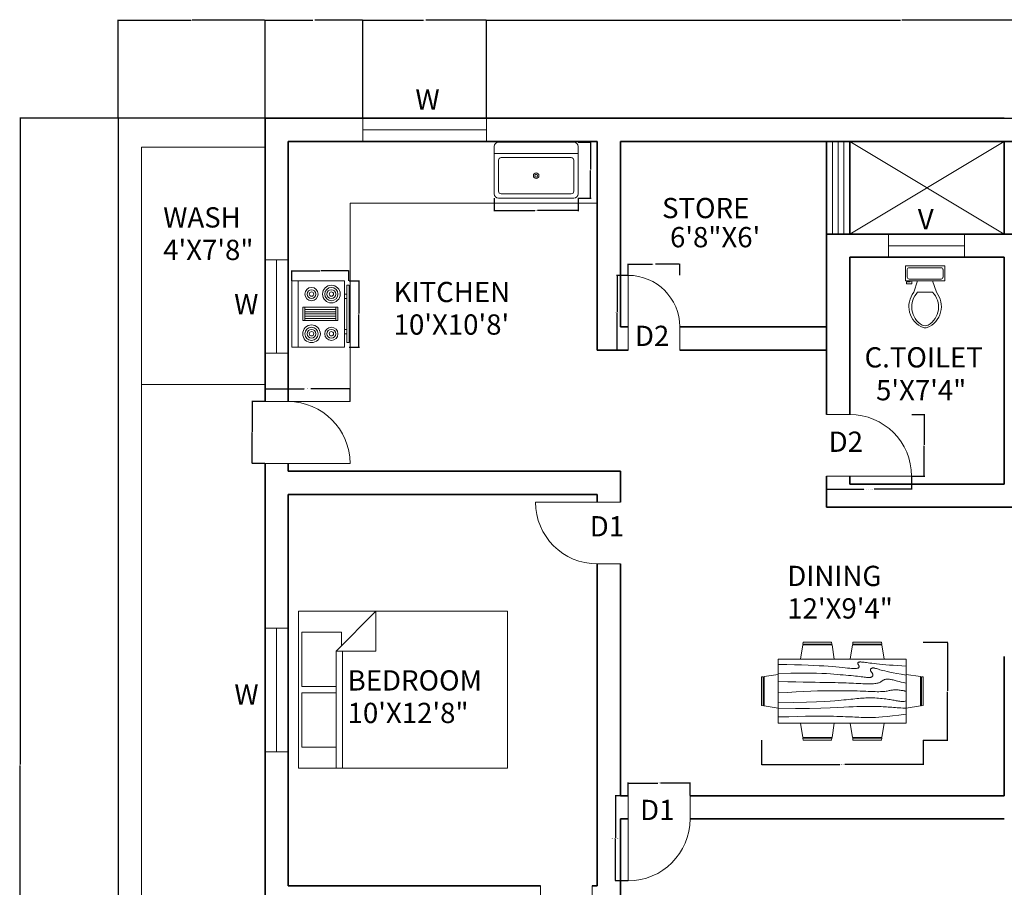
# Model space of a CAD drawing. Units: feet. Extents: x 2219 to 3039, y 1768 to 2369.
# Tile 2 of 16: x 2219 to 2601, y 2032 to 2369. Entities that reach past the tile are written whole.
import ezdxf

# ---------------------------------------------------------------- set-up
doc = ezdxf.new("R2010")
doc.units = ezdxf.units.FT
for name, color, linetype, lineweight in [('A-ANNO-DIMS', 2, 'Continuous', 18), ('A-ANNO-TEXT', 7, 'Continuous', 18), ('A-AREA-IDEN', 7, 'Continuous', 18), ('A-DOOR', 4, 'Continuous', 20), ('A-EQPM', 9, 'Continuous', 18), ('A-FLOR-CASE', 9, 'Continuous', 20), ('A-FLOR-FIXT', 9, 'Continuous', 18), ('A-FLOR-OPEN', 8, 'Continuous', 13), ('A-FURN', 8, 'Continuous', 18), ('A-GLAZ', 4, 'Continuous', 18), ('A-WALL', 7, 'Continuous', 35), ('C-PROP', 7, 'Continuous', 30), ('C-SITE', 3, 'Continuous', 20)]:
    doc.layers.add(name, color=color, linetype=linetype, lineweight=lineweight)
doc.styles.get("Standard").update_dxf_attribs({"font": 'arial.ttf'})
doc.dimstyles.get("Standard").update_dxf_attribs({"dimtxt": 0.18, "dimasz": 0.18, "dimexe": 0.18, "dimexo": 0.0625, "dimgap": 0.09, "dimtad": 0, "dimtih": 1, "dimtoh": 1, "dimdec": 4, "dimzin": 0, "dimdsep": 46, "dimtxsty": 'Standard', "dimcen": 0.09, "dimadec": 0, "dimazin": 0, "dimtfac": 1, "dimtdec": 4, "dimtofl": 0, "dimtmove": 0, "dimatfit": 3, "dimfxl": 1, "dimtolj": 1, "dimtzin": 0, "dimarcsym": 0})

# ---------------------------------------------------------------- blocks, each defined once
blk = doc.blocks.new('Toilet - top')
for p, q in [((9.5, -6), (9.5, -2)), ((-10, -8.5), (-8, -8.5)), ((-10, -9.5), (-10, -8.5)), ((-7, -9.5), (-10, -9.5)), ((-8, -8.5), (-8, -8)), ((-7, -8), (-7, -9.5)), ((-4, -8), (-6, -14)), ((4, -8), (6, -14)), ((4, -14), (-4, -14))]:
    blk.add_line(p, q)
blk.add_lwpolyline([(10.5, -8), (10.5, 0), (-10.5, 0), (-10.5, -8)], close=True)
for points in [[(-9.5, -2), (-9.5, -6)], [(8.5, -1), (-8.5, -1)], [(-8.5, -7), (8.5, -7)]]:
    blk.add_lwpolyline(points)
for centre, radius, start, end in [((-8.62, -1.88), 0.884, 81.8699, 188.1301), ((8.62, -1.88), 0.884, 351.8699, 98.1301), ((-8.62, -6.12), 0.884, 171.8699, 278.1301), ((8.62, -6.12), 0.884, 261.8699, 8.1301), ((3.52, -21.58), 12.17, 141.4691, 247.9714), ((4.2, -21.82), 11.33, 136.3677, 238.9468), ((-3.52, -21.58), 12.17, 292.0284, 38.5307), ((-4.2, -21.82), 11.33, 301.053, 43.6321), ((0, -27.88), 4, 245.7318, 294.2682), ((0, -29), 4, 254.8605, 285.1395)]:
    blk.add_arc(centre, radius, start, end)
blk = doc.blocks.new('Bed - Queen')
for p, q in [((0, -80.00003), (0, 0)), ((0, 0), (59.99999, 0)), ((59.99999, 0), (59.99999, -80.00003)), ((7.99999, -1.2), (28.79998, -1.2)), ((7.99999, -14.4), (7.99999, -1.2)), ((28.79998, -1.2), (28.79998, -14.4)), ((31.19999, -1.2), (51.99999, -1.2)), ((31.19999, -14.4), (31.19999, -1.2)), ((51.99999, -1.2), (51.99999, -16.4)), ((0, -14.4), (44.8, -14.4)), ((59.99999, -29.6), (44.8, -14.4)), ((44.8, -14.4), (44.8, -29.6)), ((44.8, -16.8), (0, -16.8)), ((51.99999, -16.4), (46.79936, -16.4)), ((44.8, -29.6), (59.99999, -29.6)), ((59.99999, -80.00003), (0, -80.00003))]:
    blk.add_line(p, q)
blk = doc.blocks.new('Dining Set - 36 x 72 in.')
for p, q in [((-22.2343, 26.00059), (-23.4847, 17.99762)), ((-22.2304, 26), (-5.7608, 26)), ((-22, 27.5), (-22.1562, 26.50042)), ((-5.8416, 26.5), (-22.1534, 26.5)), ((-22, 27.5), (-6, 27.5)), ((-5.8437, 26.49966), (-6, 27.5)), ((-4.5152, 17.99762), (-5.7655, 25.99926)), ((5.7657, 26.00059), (4.5153, 17.99762)), ((5.7696, 26), (22.2392, 26)), ((6, 27.5), (5.8438, 26.50042)), ((22.1584, 26.5), (5.8466, 26.5)), ((6, 27.5), (22, 27.5)), ((22.1563, 26.49966), (22, 27.5)), ((23.4848, 17.99762), (22.2345, 25.99926)), ((36, 18), (-36, 18)), ((-36, 18), (-36, -18)), ((36, -18), (36, 18)), ((-45.5, 8), (-44.5004, 8.15617)), ((-45.5, 8), (-45.5, -8)), ((-44.5, -8.15843), (-44.5, 8.15338)), ((-44.0006, 8.23428), (-35.9976, 9.48474)), ((-44, 8.23041), (-44, -8.23915)), ((44.0006, 8.23428), (35.9976, 9.48474)), ((44, 8.23041), (44, -8.23915)), ((44.5, -8.15843), (44.5, 8.15338)), ((45.5, 8), (44.5005, 8.15617)), ((45.5, 8), (45.5, -8)), ((-44.4997, -8.15631), (-45.5, -8)), ((-35.9976, -9.48476), (-43.9993, -8.2345)), ((35.9976, -9.48476), (43.9993, -8.2345)), ((44.4997, -8.15631), (45.5, -8)), ((-36, -18), (36, -18)), ((-22.2343, -26.0006), (-23.4847, -17.99762)), ((-4.5152, -17.99762), (-5.7655, -25.99928)), ((5.7657, -26.0006), (4.5153, -17.99762)), ((23.4848, -17.99762), (22.2345, -25.99928)), ((-22.2304, -26), (-5.7608, -26)), ((-22, -27.5), (-22.1562, -26.50044)), ((-5.8416, -26.5), (-22.1534, -26.5)), ((-22, -27.5), (-6, -27.5)), ((-5.8437, -26.49967), (-6, -27.5)), ((5.7696, -26), (22.2392, -26)), ((6, -27.5), (5.8438, -26.50044)), ((22.1584, -26.5), (5.8466, -26.5)), ((6, -27.5), (22, -27.5)), ((22.1563, -26.49967), (22, -27.5))]:
    blk.add_line(p, q)
for points in [[(-36, 15), (-31.1772, 14.97754), (-26.8079, 14.91406), (-22.8538, 14.81543), (-19.276, 14.6875), (-16.0362, 14.53613), (-13.0957, 14.36718), (-10.4159, 14.18652), (-7.9583, 14), (-5.6904, 13.81315), (-3.6035, 13.63021), (-1.6954, 13.45508), (0.0365, 13.29166), (1.5945, 13.14388), (2.9811, 13.01562), (4.1988, 12.9108), (5.25, 12.83333), (6.1393, 12.78613), (6.8802, 12.76823), (7.4883, 12.77767), (7.9792, 12.8125), (8.3685, 12.87077), (8.6719, 12.95052), (8.9049, 13.0498), (9.0833, 13.16666), (9.2205, 13.29899), (9.3216, 13.44401), (9.3895, 13.59879), (9.4271, 13.76041), (9.4373, 13.92594), (9.4232, 14.09245), (9.3875, 14.257), (9.3333, 14.41666), (9.2638, 14.56917), (9.1836, 14.71484), (9.0975, 14.85465), (9.0104, 14.98958), (8.9272, 15.1206), (8.8529, 15.2487), (8.7922, 15.37483), (8.75, 15.5), (8.7305, 15.62467), (8.7344, 15.74739), (8.7617, 15.86621), (8.8125, 15.97916), (8.8867, 16.08431), (8.9844, 16.17968), (9.1055, 16.26334), (9.25, 16.33333), (9.4189, 16.38802), (9.6172, 16.42708), (9.8506, 16.45052), (10.125, 16.45833), (10.4463, 16.45052), (10.8203, 16.42708), (11.2529, 16.38802), (11.75, 16.33333), (12.3184, 16.26318), (12.9694, 16.17838), (13.7151, 16.07991), (14.5677, 15.96875), (15.5395, 15.84586), (16.6426, 15.71224), (17.8893, 15.56884), (19.2917, 15.41666), (20.859, 15.25667), (22.5879, 15.08984), (24.4721, 14.91715), (26.5052, 14.73958), (28.6809, 14.5581), (30.9929, 14.3737), (33.4347, 14.18733), (36, 14)], [(-36, 10), (-28.9766, 10.14274), (-23.1725, 10.20442), (-18.4241, 10.19775), (-14.5677, 10.13541), (-11.4399, 10.03011), (-8.877, 9.89453), (-6.7154, 9.74137), (-4.7917, 9.58333), (-2.9698, 9.43082), (-1.2246, 9.28515), (0.4415, 9.14534), (2.026, 9.01041), (3.5266, 8.87939), (4.9408, 8.7513), (6.266, 8.62516), (7.5, 8.5), (8.6411, 8.37549), (9.6914, 8.2539), (10.6538, 8.13818), (11.5312, 8.03125), (12.3267, 7.93603), (13.043, 7.85547), (13.6831, 7.79248), (14.25, 7.75), (14.7471, 7.7303), (15.1797, 7.73307), (15.5537, 7.75732), (15.875, 7.80208), (16.1494, 7.86637), (16.3828, 7.94922), (16.5811, 8.04964), (16.75, 8.16666), (16.8944, 8.29915), (17.0143, 8.44531), (17.1089, 8.60319), (17.1771, 8.77083), (17.218, 8.94629), (17.2305, 9.1276), (17.2137, 9.31282), (17.1667, 9.5), (17.0895, 9.6875), (16.987, 9.875), (16.8649, 10.0625), (16.7292, 10.25), (16.5856, 10.4375), (16.4401, 10.625), (16.2985, 10.8125), (16.1667, 11), (16.05, 11.18733), (15.9518, 11.3737), (15.8752, 11.5581), (15.8229, 11.73958), (15.798, 11.91715), (15.8034, 12.08984), (15.842, 12.25667), (15.9167, 12.41666), (16.0295, 12.56836), (16.1784, 12.70833), (16.3605, 12.83268), (16.5729, 12.9375), (16.8127, 13.01888), (17.0768, 13.07291), (17.3625, 13.0957), (17.6667, 13.08333), (17.9894, 13.03312), (18.3418, 12.94726), (18.7382, 12.82918), (19.1927, 12.68229), (19.7195, 12.51001), (20.3327, 12.31575), (21.0465, 12.10294), (21.875, 11.875), (22.8357, 11.63354), (23.959, 11.37304), (25.2786, 11.08618), (26.8282, 10.76562), (28.6414, 10.40405), (30.752, 9.99414), (33.1936, 9.52856), (36, 9)], [(-36, 5.5), (-30.7157, 5.3348), (-26.069, 5.20963), (-21.9946, 5.11767), (-18.4271, 5.05208), (-15.3009, 5.00602), (-12.5508, 4.97265), (-10.1112, 4.94515), (-7.9167, 4.91666), (-5.909, 4.88167), (-4.0586, 4.83984), (-2.3429, 4.79215), (-0.7396, 4.73958), (0.7739, 4.6831), (2.22, 4.6237), (3.6213, 4.56233), (5, 4.5), (6.373, 4.43782), (7.7344, 4.3776), (9.0723, 4.32129), (10.375, 4.27083), (11.6309, 4.22819), (12.8281, 4.19531), (13.9551, 4.17415), (15, 4.16666), (15.954, 4.17448), (16.819, 4.19791), (17.6001, 4.23698), (18.3021, 4.29166), (18.9299, 4.36198), (19.4883, 4.44791), (19.9823, 4.54948), (20.4167, 4.66666), (20.7969, 4.79899), (21.1302, 4.94401), (21.4245, 5.09879), (21.6875, 5.26041), (21.9271, 5.42594), (22.1511, 5.59245), (22.3672, 5.757), (22.5834, 5.91666), (22.8065, 6.06868), (23.0404, 6.21093), (23.2879, 6.34147), (23.5521, 6.45833), (23.8358, 6.55957), (24.142, 6.64323), (24.4735, 6.70735), (24.8334, 6.75), (25.2235, 6.76969), (25.642, 6.76692), (26.0858, 6.74267), (26.5521, 6.69791), (27.0379, 6.63362), (27.5404, 6.55078), (28.0565, 6.45036), (28.5834, 6.33333), (29.1242, 6.19987), (29.7071, 6.04687), (30.3661, 5.87044), (31.1354, 5.66666), (32.0493, 5.43164), (33.142, 5.16146), (34.4475, 4.85221), (36, 4.5)], [(-36, -1), (-30.7915, -0.6591), (-26.0195, -0.38216), (-21.6519, -0.16284), (-17.6563, 0.00521), (-14.0005, 0.12833), (-10.6523, 0.21289), (-7.5796, 0.26522), (-4.75, 0.29166), (-2.134, 0.29793), (0.2878, 0.28711), (2.5317, 0.26163), (4.6146, 0.22396), (6.5529, 0.17651), (8.3633, 0.12174), (10.0623, 0.06209), (11.6667, 0), (13.1899, -0.06201), (14.6341, -0.1211), (15.9982, -0.17432), (17.2813, -0.21875), (18.4823, -0.25147), (19.6003, -0.26953), (20.6343, -0.27002), (21.5834, -0.25), (22.4481, -0.20768), (23.2357, -0.14584), (23.9549, -0.06836), (24.6146, 0.02083), (25.2235, 0.11784), (25.7904, 0.21875), (26.3241, 0.31966), (26.8334, 0.41666), (27.3265, 0.50618), (27.8099, 0.58593), (28.2894, 0.65397), (28.7709, 0.70833), (29.2601, 0.74707), (29.763, 0.76823), (30.2855, 0.76985), (30.8334, 0.75), (31.4088, 0.70784), (31.9994, 0.64713), (32.589, 0.57275), (33.1615, 0.48958), (33.7008, 0.4025), (34.1908, 0.3164), (34.6153, 0.23616), (34.9584, 0.16666), (35.2099, 0.11165), (35.3848, 0.07031), (35.504, 0.04069), (35.5886, 0.02083), (35.6594, 0.00879), (35.7377, 0.0026), (35.8442, 0.00032), (36, 0)], [(-36, -6.5), (-27.1843, -6.31267), (-20.084, -6.1263), (-14.469, -5.9419), (-10.1094, -5.76042), (-6.7752, -5.58285), (-4.2363, -5.41016), (-2.2629, -5.24333), (-0.625, -5.08334), (0.8708, -4.93099), (2.2715, -4.78646), (3.5872, -4.64974), (4.8281, -4.52084), (6.0046, -4.39974), (7.127, -4.28646), (8.2053, -4.18099), (9.25, -4.08334), (10.2705, -3.99382), (11.2734, -3.91407), (12.2647, -3.84603), (13.25, -3.79167), (14.2354, -3.75293), (15.2266, -3.73177), (16.2295, -3.73015), (17.25, -3.75), (18.2912, -3.79248), (19.3451, -3.85547), (20.4009, -3.93604), (21.4479, -4.03125), (22.4754, -4.13819), (23.4727, -4.25391), (24.4289, -4.37549), (25.3334, -4.5), (26.1785, -4.62492), (26.9694, -4.74935), (27.7145, -4.87281), (28.4219, -4.99479), (29.1, -5.11483), (29.7572, -5.23242), (30.4016, -5.34709), (31.0417, -5.45834), (31.6837, -5.56437), (32.3262, -5.65821), (32.9658, -5.73153), (33.599, -5.77604), (34.2224, -5.78345), (34.8327, -5.74545), (35.4264, -5.65373), (36, -5.5)], [(-36, -10), (-26.4022, -9.81299), (-18.4675, -9.62891), (-11.9839, -9.45069), (-6.7396, -9.28125), (-2.5226, -9.12354), (0.8789, -8.98047), (3.6769, -8.85498), (6.0833, -8.75), (8.2767, -8.66765), (10.3021, -8.60677), (12.1712, -8.56543), (13.8958, -8.54167), (15.4876, -8.53353), (16.9583, -8.53907), (18.3197, -8.55632), (19.5834, -8.58334), (20.7616, -8.61841), (21.8685, -8.66081), (22.9188, -8.71004), (23.9271, -8.76563), (24.9081, -8.82707), (25.8763, -8.89388), (26.8465, -8.96558), (27.8334, -9.04167), (28.8474, -9.12118), (29.8828, -9.20117), (30.93, -9.27824), (31.9792, -9.34896), (33.0205, -9.40991), (34.0443, -9.45768), (35.0407, -9.48885), (36, -9.5)], [(-36, -14.5), (-30.0881, -14.33513), (-25.0332, -14.21224), (-20.7312, -14.12647), (-17.0781, -14.07292), (-13.97, -14.04671), (-11.3027, -14.04297), (-8.9724, -14.05681), (-6.875, -14.08334), (-4.9224, -14.11833), (-3.0905, -14.16016), (-1.3709, -14.20785), (0.2448, -14.26042), (1.7647, -14.3169), (3.1973, -14.3763), (4.5507, -14.43767), (5.8333, -14.5), (7.0554, -14.5621), (8.235, -14.62175), (9.3922, -14.67652), (10.5469, -14.72396), (11.7192, -14.76164), (12.929, -14.78711), (14.1965, -14.79794), (15.5417, -14.79167), (16.9933, -14.76424), (18.6152, -14.70508), (20.4804, -14.60197), (22.6615, -14.44271), (25.2312, -14.21509), (28.2624, -13.9069), (31.8277, -13.50594), (36, -13)]]:
    blk.add_lwpolyline(points)
blk = doc.blocks.new('Sink-single - 30 in top')
blk.add_line((-15, -3.999996), (15, -3.999996))
for points in [[(-13.5, 0), (13.5, 0)], [(-15, -18.499996), (-15, -1.5)], [(15, -1.5), (15, -18.499996)], [(-13.5, -17.499996), (-13.5, -6.499996)], [(-12.5, -5.499996), (12.5, -5.499996)], [(13.5, -6.499996), (13.5, -17.499996)], [(13.5, -19.999996), (-13.5, -19.999996)], [(12.5, -18.499996), (-12.5, -18.499996)]]:
    blk.add_lwpolyline(points)
for radius in [1, 0.5]:
    blk.add_circle((0, -11.999996), radius)
for centre, radius, start, end in [((-13.5, -1.5), 1.5, 90, 180), ((13.5, -1.5), 1.5, 0, 90), ((-12.5, -6.499996), 1, 90, 180), ((12.5, -6.499996), 1, 0, 90), ((-12.5, -17.499996), 1, 180, 270), ((12.5, -17.499996), 1, 270, 0), ((-13.5, -18.499996), 1.5, 180, 270), ((13.5, -18.499996), 1.5, 270, 0)]:
    blk.add_arc(centre, radius, start, end)
blk = doc.blocks.new('Range-Oven - 30 in top')
for p, q in [((0, -3), (30, -3)), ((12, -6), (18, -6)), ((13, -20), (13, -6)), ((14, -6), (14, -20)), ((15, -20), (15, -6)), ((16, -6), (16, -20)), ((17, -20), (17, -6)), ((18, -20), (12, -20)), ((6, -24), (6, -25)), ((8, -25), (8, -24)), ((22, -25), (22, -24)), ((24, -24), (24, -25))]:
    blk.add_line(p, q)
for points in [[(0, -24), (0, 0), (30, 0), (30, -24)], [(12, -21), (12, -5), (18, -5), (18, -21)], [(2, -26), (2, -25), (28, -25), (28, -26)]]:
    blk.add_lwpolyline(points, close=True)
for centre, radius in [((6, -9), 4), ((6, -9), 3), ((6, -9), 2), ((6, -9), 1), ((24, -9), 3), ((24, -9), 2), ((24, -9), 1), ((6, -18), 3), ((6, -18), 2), ((6, -18), 1), ((24, -18), 4), ((24, -18), 3), ((24, -18), 2), ((24, -18), 1)]:
    blk.add_circle(centre, radius)
blk = doc.blocks.new('DOOR-24-LEAF')
blk.add_line((33, 0), (0, 0))
blk.add_arc((9, 0), 24, 0, 90)
blk = doc.blocks.new('DOOR-24-INTEGRAL-JAMB')
for p, q in [((9, 24), (0, 24)), ((33, 0), (0, 0))]:
    blk.add_line(p, q)
blk.add_arc((9, 0), 24, 0, 90)
blk = doc.blocks.new('DOOR-24-SPLIT-JAMB')
for p, q in [((0, 24), (0, 33)), ((24, 24), (24, 33)), ((0, 24), (0, 0))]:
    blk.add_line(p, q)
blk.add_arc((0, 24), 24, 270, 0)
blk = doc.blocks.new('DOOR-20')
for p, q in [((0, 29), (0, 0)), ((20, 9), (20, 0))]:
    blk.add_line(p, q)
blk.add_arc((0, 9), 20, 0, 90)
blk = doc.blocks.new('WINDOW-48')
for p, q in [((0, 9), (0, 0)), ((48, 9), (48, 0)), ((0, 4.5), (48, 4.5))]:
    blk.add_line(p, q)
blk = doc.blocks.new('*D16')
at = {"layer": 'A-ANNO-DIMS', "color": 0, "lineweight": -2, "transparency": 16777216}
for p, q in [((2532.4, 2191.86), (2532.4, 2186.79)), ((2565.4, 2191.86), (2565.4, 2186.79)), ((2532.58, 2186.97), (2546.92, 2186.97)), ((2565.22, 2186.97), (2550.87, 2186.97))]:
    blk.add_line(p, q, dxfattribs=at)
at = {"layer": 'A-ANNO-DIMS', "color": 0, "transparency": 16777216}
for points in [[(2532.58, 2187), (2532.58, 2186.94), (2532.4, 2186.97)], [(2565.22, 2187), (2565.22, 2186.94), (2565.4, 2186.97)]]:
    blk.add_solid(points, dxfattribs=at)
at = {"layer": 'Defpoints', "color": 0, "transparency": 16777216}
for p in [(2532.4, 2191.92), (2565.4, 2191.92), (2565.4, 2186.97)]:
    blk.add_point(p, dxfattribs=at)
at = {"layer": 'A-ANNO-DIMS', "color": 0, "transparency": 16777216, "insert": (2548.9, 2186.97), "char_height": 0.18, "attachment_point": 5}
blk.add_mtext('\\A1;INTEGRAL-JAMB DOOR 33 TYP.', dxfattribs=at)
blk = doc.blocks.new('*D17')
at = {"layer": 'A-ANNO-DIMS', "color": 0, "lineweight": -2, "transparency": 16777216}
for p, q in [((2565.46, 2215.92), (2570.53, 2215.92)), ((2570.35, 2215.74), (2570.35, 2204.1)), ((2570.35, 2192.1), (2570.35, 2203.74)), ((2565.46, 2191.92), (2570.53, 2191.92))]:
    blk.add_line(p, q, dxfattribs=at)
at = {"layer": 'A-ANNO-DIMS', "color": 0, "transparency": 16777216}
for points in [[(2570.32, 2215.74), (2570.38, 2215.74), (2570.35, 2215.92)], [(2570.32, 2192.1), (2570.38, 2192.1), (2570.35, 2191.92)]]:
    blk.add_solid(points, dxfattribs=at)
at = {"layer": 'Defpoints', "color": 0, "transparency": 16777216}
for p in [(2565.4, 2215.92), (2570.35, 2215.92), (2565.4, 2191.92)]:
    blk.add_point(p, dxfattribs=at)
at = {"layer": 'A-ANNO-DIMS', "color": 0, "transparency": 16777216, "insert": (2570.35, 2203.92), "char_height": 0.18, "attachment_point": 5}
blk.add_mtext('\\A1;24 TYP.', dxfattribs=at)
blk = doc.blocks.new('*D22')
at = {"layer": 'A-ANNO-DIMS', "color": 0, "lineweight": -2, "transparency": 16777216}
for p, q in [((2314.4, 2220.99), (2314.4, 2226.05)), ((2314.58, 2225.87), (2329.61, 2225.87)), ((2347.22, 2225.87), (2332.18, 2225.87)), ((2347.4, 2220.99), (2347.4, 2226.05))]:
    blk.add_line(p, q, dxfattribs=at)
at = {"layer": 'A-ANNO-DIMS', "color": 0, "transparency": 16777216}
for points in [[(2314.58, 2225.9), (2314.58, 2225.84), (2314.4, 2225.87)], [(2347.22, 2225.9), (2347.22, 2225.84), (2347.4, 2225.87)]]:
    blk.add_solid(points, dxfattribs=at)
at = {"layer": 'Defpoints', "color": 0, "transparency": 16777216}
for p in [(2347.4, 2225.87), (2314.4, 2220.92), (2347.4, 2220.92)]:
    blk.add_point(p, dxfattribs=at)
at = {"layer": 'A-ANNO-DIMS', "color": 0, "transparency": 16777216, "insert": (2330.9, 2225.87), "char_height": 0.18, "attachment_point": 5}
blk.add_mtext('\\A1;DOOR LEAF 33 TYP.', dxfattribs=at)
blk = doc.blocks.new('*D23')
at = {"layer": 'A-ANNO-DIMS', "color": 0, "lineweight": -2, "transparency": 16777216}
for p, q in [((2314.34, 2220.92), (2309.27, 2220.92)), ((2309.45, 2220.74), (2309.45, 2209.1)), ((2309.45, 2197.1), (2309.45, 2208.74)), ((2314.34, 2196.92), (2309.27, 2196.92))]:
    blk.add_line(p, q, dxfattribs=at)
at = {"layer": 'A-ANNO-DIMS', "color": 0, "transparency": 16777216}
for points in [[(2309.42, 2220.74), (2309.48, 2220.74), (2309.45, 2220.92)], [(2309.42, 2197.1), (2309.48, 2197.1), (2309.45, 2196.92)]]:
    blk.add_solid(points, dxfattribs=at)
at = {"layer": 'Defpoints', "color": 0, "transparency": 16777216}
for p in [(2309.45, 2220.92), (2314.4, 2220.92), (2314.4, 2196.92)]:
    blk.add_point(p, dxfattribs=at)
at = {"layer": 'A-ANNO-DIMS', "color": 0, "transparency": 16777216, "insert": (2309.45, 2208.92), "char_height": 0.18, "attachment_point": 5}
blk.add_mtext('\\A1;24 TYP.', dxfattribs=at)
blk = doc.blocks.new('*D30')
at = {"layer": 'A-ANNO-DIMS', "color": 0, "lineweight": -2, "transparency": 16777216}
for p, q in [((2455.34, 2067.92), (2450.27, 2067.92)), ((2450.45, 2067.74), (2450.45, 2051.61)), ((2450.45, 2035.1), (2450.45, 2051.24)), ((2455.34, 2034.92), (2450.27, 2034.92))]:
    blk.add_line(p, q, dxfattribs=at)
at = {"layer": 'A-ANNO-DIMS', "color": 0, "transparency": 16777216}
for points in [[(2450.42, 2067.74), (2450.48, 2067.74), (2450.45, 2067.92)], [(2450.42, 2035.1), (2450.48, 2035.1), (2450.45, 2034.92)]]:
    blk.add_solid(points, dxfattribs=at)
at = {"layer": 'Defpoints', "color": 0, "transparency": 16777216}
for p in [(2450.45, 2067.92), (2455.4, 2067.92), (2455.4, 2034.92)]:
    blk.add_point(p, dxfattribs=at)
at = {"layer": 'A-ANNO-DIMS', "color": 0, "transparency": 16777216, "insert": (2450.45, 2051.42), "char_height": 0.18, "attachment_point": 5}
blk.add_mtext('\\A1;SPLIT-JAMB DOOR 33 TYP.', dxfattribs=at)
blk = doc.blocks.new('*D31')
at = {"layer": 'A-ANNO-DIMS', "color": 0, "lineweight": -2, "transparency": 16777216}
for p, q in [((2455.4, 2067.99), (2455.4, 2073.05)), ((2455.58, 2072.87), (2466.87, 2072.87)), ((2479.22, 2072.87), (2467.93, 2072.87)), ((2479.4, 2067.99), (2479.4, 2073.05))]:
    blk.add_line(p, q, dxfattribs=at)
at = {"layer": 'A-ANNO-DIMS', "color": 0, "transparency": 16777216}
for points in [[(2455.58, 2072.9), (2455.58, 2072.84), (2455.4, 2072.87)], [(2479.22, 2072.9), (2479.22, 2072.84), (2479.4, 2072.87)]]:
    blk.add_solid(points, dxfattribs=at)
at = {"layer": 'Defpoints', "color": 0, "transparency": 16777216}
for p in [(2479.4, 2072.87), (2455.4, 2067.92), (2479.4, 2067.92)]:
    blk.add_point(p, dxfattribs=at)
at = {"layer": 'A-ANNO-DIMS', "color": 0, "transparency": 16777216, "insert": (2467.4, 2072.87), "char_height": 0.18, "attachment_point": 5}
blk.add_mtext('\\A1;24 TYP.', dxfattribs=at)
blk = doc.blocks.new('*D32')
at = {"layer": 'A-ANNO-DIMS', "color": 0, "lineweight": -2, "transparency": 16777216}
for p, q in [((2455.34, 2269.92), (2450.87, 2269.92)), ((2451.05, 2269.74), (2451.05, 2255.61)), ((2451.05, 2241.1), (2451.05, 2255.24)), ((2455.34, 2240.92), (2450.87, 2240.92))]:
    blk.add_line(p, q, dxfattribs=at)
at = {"layer": 'A-ANNO-DIMS', "color": 0, "transparency": 16777216}
for points in [[(2451.02, 2269.74), (2451.08, 2269.74), (2451.05, 2269.92)], [(2451.02, 2241.1), (2451.08, 2241.1), (2451.05, 2240.92)]]:
    blk.add_solid(points, dxfattribs=at)
at = {"layer": 'Defpoints', "color": 0, "transparency": 16777216}
for p in [(2451.05, 2269.92), (2455.4, 2269.92), (2455.4, 2240.92)]:
    blk.add_point(p, dxfattribs=at)
at = {"layer": 'A-ANNO-DIMS', "color": 0, "transparency": 16777216, "insert": (2451.05, 2255.42), "char_height": 0.18, "attachment_point": 5}
blk.add_mtext('\\A1;DOOR 29 TYP.', dxfattribs=at)
blk = doc.blocks.new('*D33')
at = {"layer": 'A-ANNO-DIMS', "color": 0, "lineweight": -2, "transparency": 16777216}
for p, q in [((2455.4, 2269.99), (2455.4, 2274.45)), ((2475.4, 2269.99), (2475.4, 2274.45)), ((2455.58, 2274.27), (2464.87, 2274.27)), ((2475.22, 2274.27), (2465.93, 2274.27))]:
    blk.add_line(p, q, dxfattribs=at)
at = {"layer": 'A-ANNO-DIMS', "color": 0, "transparency": 16777216}
for points in [[(2455.58, 2274.3), (2455.58, 2274.24), (2455.4, 2274.27)], [(2475.22, 2274.3), (2475.22, 2274.24), (2475.4, 2274.27)]]:
    blk.add_solid(points, dxfattribs=at)
at = {"layer": 'Defpoints', "color": 0, "transparency": 16777216}
for p in [(2475.4, 2274.27), (2455.4, 2269.92), (2475.4, 2269.92)]:
    blk.add_point(p, dxfattribs=at)
at = {"layer": 'A-ANNO-DIMS', "color": 0, "transparency": 16777216, "insert": (2465.4, 2274.27), "char_height": 0.18, "attachment_point": 5}
blk.add_mtext('\\A1;20 TYP.', dxfattribs=at)
blk = doc.blocks.new('*D40')
at = {"layer": 'A-ANNO-DIMS', "color": 0, "lineweight": -2, "transparency": 16777216}
for p, q in [((2507.1, 2089.47), (2507.1, 2079.94)), ((2569.9, 2089.47), (2569.9, 2079.94)), ((2507.28, 2080.12), (2537.53, 2080.12)), ((2569.72, 2080.12), (2539.47, 2080.12))]:
    blk.add_line(p, q, dxfattribs=at)
at = {"layer": 'A-ANNO-DIMS', "color": 0, "transparency": 16777216}
for points in [[(2507.28, 2080.15), (2507.28, 2080.09), (2507.1, 2080.12)], [(2569.72, 2080.15), (2569.72, 2080.09), (2569.9, 2080.12)]]:
    blk.add_solid(points, dxfattribs=at)
at = {"layer": 'Defpoints', "color": 0, "transparency": 16777216}
for p in [(2507.1, 2089.54), (2569.9, 2089.54), (2569.9, 2080.12)]:
    blk.add_point(p, dxfattribs=at)
at = {"layer": 'A-ANNO-DIMS', "color": 0, "transparency": 16777216, "insert": (2538.5, 2080.12), "char_height": 0.18, "attachment_point": 5}
blk.add_mtext('\\A1;DINING SET 63', dxfattribs=at)
blk = doc.blocks.new('*D41')
at = {"layer": 'A-ANNO-DIMS', "color": 0, "lineweight": -2, "transparency": 16777216}
for p, q in [((2569.96, 2127.49), (2579.5, 2127.49)), ((2579.32, 2127.31), (2579.32, 2108.7)), ((2579.32, 2089.72), (2579.32, 2108.33)), ((2569.96, 2089.54), (2579.5, 2089.54))]:
    blk.add_line(p, q, dxfattribs=at)
at = {"layer": 'A-ANNO-DIMS', "color": 0, "transparency": 16777216}
for points in [[(2579.29, 2127.31), (2579.35, 2127.31), (2579.32, 2127.49)], [(2579.29, 2089.72), (2579.35, 2089.72), (2579.32, 2089.54)]]:
    blk.add_solid(points, dxfattribs=at)
at = {"layer": 'Defpoints', "color": 0, "transparency": 16777216}
for p in [(2569.9, 2127.49), (2579.32, 2127.49), (2569.9, 2089.54)]:
    blk.add_point(p, dxfattribs=at)
at = {"layer": 'A-ANNO-DIMS', "color": 0, "transparency": 16777216, "insert": (2579.32, 2108.51), "char_height": 0.18, "attachment_point": 5}
blk.add_mtext('\\A1;38', dxfattribs=at)
blk = doc.blocks.new('*D42')
at = {"layer": 'A-ANNO-DIMS', "color": 0, "lineweight": -2, "transparency": 16777216}
for p, q in [((2403.39, 2299.87), (2403.39, 2294.87)), ((2435.92, 2299.87), (2435.92, 2294.87)), ((2403.57, 2295.05), (2419.11, 2295.05)), ((2435.74, 2295.05), (2420.21, 2295.05))]:
    blk.add_line(p, q, dxfattribs=at)
at = {"layer": 'A-ANNO-DIMS', "color": 0, "transparency": 16777216}
for points in [[(2403.57, 2295.08), (2403.57, 2295.02), (2403.39, 2295.05)], [(2435.74, 2295.08), (2435.74, 2295.02), (2435.92, 2295.05)]]:
    blk.add_solid(points, dxfattribs=at)
at = {"layer": 'Defpoints', "color": 0, "transparency": 16777216}
for p in [(2403.39, 2299.93), (2435.92, 2299.93), (2435.92, 2295.05)]:
    blk.add_point(p, dxfattribs=at)
at = {"layer": 'A-ANNO-DIMS', "color": 0, "transparency": 16777216, "insert": (2419.66, 2295.05), "char_height": 0.18, "attachment_point": 5}
blk.add_mtext('\\A1;SINK 33', dxfattribs=at)
blk = doc.blocks.new('*D43')
at = {"layer": 'A-ANNO-DIMS', "color": 0, "lineweight": -2, "transparency": 16777216}
for p, q in [((2435.99, 2321.62), (2440.98, 2321.62)), ((2440.8, 2321.44), (2440.8, 2310.96)), ((2440.8, 2300.11), (2440.8, 2310.6)), ((2435.99, 2299.93), (2440.98, 2299.93))]:
    blk.add_line(p, q, dxfattribs=at)
at = {"layer": 'A-ANNO-DIMS', "color": 0, "transparency": 16777216}
for points in [[(2440.77, 2321.44), (2440.83, 2321.44), (2440.8, 2321.62)], [(2440.77, 2300.11), (2440.83, 2300.11), (2440.8, 2299.93)]]:
    blk.add_solid(points, dxfattribs=at)
at = {"layer": 'Defpoints', "color": 0, "transparency": 16777216}
for p in [(2435.92, 2321.62), (2440.8, 2321.62), (2435.92, 2299.93)]:
    blk.add_point(p, dxfattribs=at)
at = {"layer": 'A-ANNO-DIMS', "color": 0, "transparency": 16777216, "insert": (2440.8, 2310.78), "char_height": 0.18, "attachment_point": 5}
blk.add_mtext('\\A1;22', dxfattribs=at)
blk = doc.blocks.new('*D44')
at = {"layer": 'A-ANNO-DIMS', "color": 0, "lineweight": -2, "transparency": 16777216}
for p, q in [((2347.06, 2267.79), (2351.03, 2267.79)), ((2350.85, 2267.61), (2350.85, 2255.13)), ((2350.85, 2242.29), (2350.85, 2254.77)), ((2347.06, 2242.11), (2351.03, 2242.11))]:
    blk.add_line(p, q, dxfattribs=at)
at = {"layer": 'A-ANNO-DIMS', "color": 0, "transparency": 16777216}
for points in [[(2350.82, 2267.61), (2350.88, 2267.61), (2350.85, 2267.79)], [(2350.82, 2242.29), (2350.88, 2242.29), (2350.85, 2242.11)]]:
    blk.add_solid(points, dxfattribs=at)
at = {"layer": 'Defpoints', "color": 0, "transparency": 16777216}
for p in [(2346.99, 2267.79), (2350.85, 2267.79), (2346.99, 2242.11)]:
    blk.add_point(p, dxfattribs=at)
at = {"layer": 'A-ANNO-DIMS', "color": 0, "transparency": 16777216, "insert": (2350.85, 2254.95), "char_height": 0.18, "attachment_point": 5}
blk.add_mtext('\\A1;RANGE 26', dxfattribs=at)
blk = doc.blocks.new('*D45')
at = {"layer": 'A-ANNO-DIMS', "color": 0, "lineweight": -2, "transparency": 16777216}
for p, q in [((2324.74, 2267.85), (2324.74, 2271.82)), ((2324.92, 2271.64), (2335.65, 2271.64)), ((2346.81, 2271.64), (2336.09, 2271.64)), ((2346.99, 2267.85), (2346.99, 2271.82))]:
    blk.add_line(p, q, dxfattribs=at)
at = {"layer": 'A-ANNO-DIMS', "color": 0, "transparency": 16777216}
for points in [[(2324.92, 2271.67), (2324.92, 2271.61), (2324.74, 2271.64)], [(2346.81, 2271.67), (2346.81, 2271.61), (2346.99, 2271.64)]]:
    blk.add_solid(points, dxfattribs=at)
at = {"layer": 'Defpoints', "color": 0, "transparency": 16777216}
for p in [(2324.74, 2271.64), (2324.74, 2267.79), (2346.99, 2267.79)]:
    blk.add_point(p, dxfattribs=at)
at = {"layer": 'A-ANNO-DIMS', "color": 0, "transparency": 16777216, "insert": (2335.87, 2271.64), "char_height": 0.18, "attachment_point": 5}
blk.add_mtext('\\A1;22', dxfattribs=at)
blk = doc.blocks.new('*D47')
at = {"layer": 'A-ANNO-DIMS', "color": 0, "lineweight": -2, "transparency": 16777216}
for p, q in [((2257.34, 2330.92), (2219.17, 2330.92)), ((2219.35, 2330.74), (2219.35, 2080.1)), ((2219.35, 1829.1), (2219.35, 2079.74)), ((2257.34, 1828.92), (2219.17, 1828.92))]:
    blk.add_line(p, q, dxfattribs=at)
at = {"layer": 'A-ANNO-DIMS', "color": 0, "transparency": 16777216}
for points in [[(2219.32, 2330.74), (2219.38, 2330.74), (2219.35, 2330.92)], [(2219.32, 1829.1), (2219.38, 1829.1), (2219.35, 1828.92)]]:
    blk.add_solid(points, dxfattribs=at)
at = {"layer": 'Defpoints', "color": 0, "transparency": 16777216}
for p in [(2219.35, 2330.92), (2257.4, 2330.92), (2257.4, 1828.92)]:
    blk.add_point(p, dxfattribs=at)
at = {"layer": 'A-ANNO-DIMS', "color": 0, "transparency": 16777216, "insert": (2219.35, 2079.92), "char_height": 0.18, "attachment_point": 5}
blk.add_mtext('\\A1;502', dxfattribs=at)
blk = doc.blocks.new('*D52')
at = {"layer": 'A-ANNO-DIMS', "color": 0, "lineweight": -2, "transparency": 16777216}
for p, q in [((2257.4, 2330.99), (2257.4, 2369.15)), ((2257.58, 2368.97), (2285.68, 2368.97)), ((2314.22, 2368.97), (2286.12, 2368.97)), ((2314.4, 2330.99), (2314.4, 2369.15))]:
    blk.add_line(p, q, dxfattribs=at)
at = {"layer": 'A-ANNO-DIMS', "color": 0, "transparency": 16777216}
for points in [[(2257.58, 2369), (2257.58, 2368.94), (2257.4, 2368.97)], [(2314.22, 2369), (2314.22, 2368.94), (2314.4, 2368.97)]]:
    blk.add_solid(points, dxfattribs=at)
at = {"layer": 'Defpoints', "color": 0, "transparency": 16777216}
for p in [(2314.4, 2368.97), (2257.4, 2330.92), (2314.4, 2330.92)]:
    blk.add_point(p, dxfattribs=at)
at = {"layer": 'A-ANNO-DIMS', "color": 0, "transparency": 16777216, "insert": (2285.9, 2368.97), "char_height": 0.18, "attachment_point": 5}
blk.add_mtext('\\A1;57', dxfattribs=at)
blk = doc.blocks.new('*D53')
at = {"layer": 'A-ANNO-DIMS', "color": 0, "lineweight": -2, "transparency": 16777216}
for p, q in [((2314.4, 2330.99), (2314.4, 2369.15)), ((2314.58, 2368.97), (2332.98, 2368.97)), ((2352.17, 2368.97), (2333.77, 2368.97)), ((2352.35, 2330.99), (2352.35, 2369.15))]:
    blk.add_line(p, q, dxfattribs=at)
at = {"layer": 'A-ANNO-DIMS', "color": 0, "transparency": 16777216}
for points in [[(2314.58, 2369), (2314.58, 2368.94), (2314.4, 2368.97)], [(2352.17, 2369), (2352.17, 2368.94), (2352.35, 2368.97)]]:
    blk.add_solid(points, dxfattribs=at)
at = {"layer": 'Defpoints', "color": 0, "transparency": 16777216}
for p in [(2352.35, 2368.97), (2314.4, 2330.92), (2352.35, 2330.92)]:
    blk.add_point(p, dxfattribs=at)
at = {"layer": 'A-ANNO-DIMS', "color": 0, "transparency": 16777216, "insert": (2333.37, 2368.97), "char_height": 0.18, "attachment_point": 5}
blk.add_mtext('\\A1;37.95', dxfattribs=at)
blk = doc.blocks.new('*D54')
at = {"layer": 'A-ANNO-DIMS', "color": 0, "lineweight": -2, "transparency": 16777216}
for p, q in [((2352.35, 2330.99), (2352.35, 2369.15)), ((2352.53, 2368.97), (2375.97, 2368.97)), ((2400.2, 2368.97), (2376.76, 2368.97)), ((2400.38, 2330.99), (2400.38, 2369.15))]:
    blk.add_line(p, q, dxfattribs=at)
at = {"layer": 'A-ANNO-DIMS', "color": 0, "transparency": 16777216}
for points in [[(2352.53, 2369), (2352.53, 2368.94), (2352.35, 2368.97)], [(2400.2, 2369), (2400.2, 2368.94), (2400.38, 2368.97)]]:
    blk.add_solid(points, dxfattribs=at)
at = {"layer": 'Defpoints', "color": 0, "transparency": 16777216}
for p in [(2400.38, 2368.97), (2352.35, 2330.92), (2400.38, 2330.92)]:
    blk.add_point(p, dxfattribs=at)
at = {"layer": 'A-ANNO-DIMS', "color": 0, "transparency": 16777216, "insert": (2376.37, 2368.97), "char_height": 0.18, "attachment_point": 5}
blk.add_mtext('\\A1;48.03', dxfattribs=at)
blk = doc.blocks.new('*D55')
at = {"layer": 'A-ANNO-DIMS', "color": 0, "lineweight": -2, "transparency": 16777216}
for p, q in [((2400.38, 2330.99), (2400.38, 2369.15)), ((2400.56, 2368.97), (2561.1, 2368.97)), ((2722.22, 2368.97), (2561.68, 2368.97)), ((2722.4, 2330.99), (2722.4, 2369.15))]:
    blk.add_line(p, q, dxfattribs=at)
at = {"layer": 'A-ANNO-DIMS', "color": 0, "transparency": 16777216}
for points in [[(2400.56, 2369), (2400.56, 2368.94), (2400.38, 2368.97)], [(2722.22, 2369), (2722.22, 2368.94), (2722.4, 2368.97)]]:
    blk.add_solid(points, dxfattribs=at)
at = {"layer": 'Defpoints', "color": 0, "transparency": 16777216}
for p in [(2722.4, 2368.97), (2400.38, 2330.92), (2722.4, 2330.92)]:
    blk.add_point(p, dxfattribs=at)
at = {"layer": 'A-ANNO-DIMS', "color": 0, "transparency": 16777216, "insert": (2561.39, 2368.97), "char_height": 0.18, "attachment_point": 5}
blk.add_mtext('\\A1;322', dxfattribs=at)

msp = doc.modelspace()

# ---------------------------------------------------------------- linework, layer by layer
at = {"layer": 'A-FLOR-CASE'}
for p, q in [((2347.4, 2297.923), (2443.4, 2297.923)), ((2347.4, 2220.923), (2347.4, 2297.923)), ((2347.4, 2220.923), (2314.4, 2220.923))]:
    msp.add_line(p, q, dxfattribs=at)
at = {"layer": 'A-FLOR-OPEN'}
for p, q in [((2534.65, 2321.923), (2534.65, 2285.923)), ((2536.9, 2321.923), (2536.9, 2285.923)), ((2539.15, 2321.923), (2539.15, 2285.923)), ((2541.4, 2321.923), (2601.4, 2285.923)), ((2601.4, 2321.923), (2541.4, 2285.923))]:
    msp.add_line(p, q, dxfattribs=at)
at = {"layer": 'A-GLAZ'}
for p, q in [((2352.35, 2330.923), (2352.35, 2321.923)), ((2400.382, 2321.923), (2400.382, 2330.923)), ((2352.35, 2326.423), (2400.382, 2326.423)), ((2556.379, 2285.923), (2556.379, 2276.923)), ((2585.985, 2285.923), (2585.985, 2276.923)), ((2556.379, 2281.423), (2585.985, 2281.423)), ((2314.4, 2275.923), (2323.4, 2275.923)), ((2318.9, 2275.923), (2318.9, 2239.71)), ((2323.4, 2239.71), (2314.4, 2239.71))]:
    msp.add_line(p, q, dxfattribs=at)
at = {"layer": 'A-WALL'}
for p, q in [((2314.4, 2330.923), (2443.4, 2330.923)), ((2314.4, 2330.923), (2532.4, 2330.923)), ((2314.4, 2330.923), (2601.4, 2330.923)), ((2314.4, 2220.923), (2314.4, 2330.923)), ((2323.4, 2321.923), (2443.4, 2321.923)), ((2323.4, 2220.923), (2323.4, 2321.923)), ((2443.4, 2321.923), (2443.4, 2240.923)), ((2452.4, 2321.923), (2452.4, 2249.923)), ((2452.4, 2321.923), (2532.4, 2321.923)), ((2532.4, 2321.923), (2532.4, 2249.923)), ((2532.4, 2321.923), (2610.4, 2321.923)), ((2541.4, 2321.923), (2541.4, 2285.923)), ((2601.4, 2321.923), (2601.4, 2285.923)), ((2601.4, 2285.923), (2601.4, 2321.923)), ((2610.4, 2285.923), (2532.4, 2285.923)), ((2532.4, 2215.923), (2532.4, 2276.923)), ((2601.4, 2276.923), (2541.4, 2276.923)), ((2541.4, 2276.923), (2541.4, 2249.923)), ((2541.4, 2215.923), (2541.4, 2276.923)), ((2601.4, 2276.923), (2601.4, 2188.923)), ((2601.4, 2188.923), (2601.4, 2276.923)), ((2455.4, 2249.923), (2452.4, 2249.923)), ((2532.4, 2249.923), (2475.4, 2249.923)), ((2455.4, 2240.923), (2443.4, 2240.923)), ((2532.4, 2240.923), (2475.4, 2240.923)), ((2314.4, 1897.923), (2314.4, 2196.923)), ((2323.4, 2193.923), (2323.4, 2196.923)), ((2452.4, 2193.923), (2323.4, 2193.923)), ((2452.4, 2193.923), (2452.4, 2181.923)), ((2532.4, 2179.923), (2532.4, 2191.923)), ((2541.4, 2188.923), (2541.4, 2191.923)), ((2601.4, 2188.923), (2541.4, 2188.923)), ((2314.4, 2184.923), (2314.4, 2032.923)), ((2443.4, 2184.923), (2323.4, 2184.923)), ((2323.4, 2184.923), (2323.4, 2032.923)), ((2443.4, 2181.923), (2443.4, 2184.923)), ((2452.4, 2181.923), (2452.4, 2184.923)), ((2610.4, 2179.923), (2532.4, 2179.923)), ((2443.4, 2032.923), (2443.4, 2157.923)), ((2452.4, 2157.923), (2452.4, 2067.923)), ((2452.4, 2067.923), (2452.4, 2157.923)), ((2601.4, 2067.923), (2601.4, 2121.923)), ((2455.4, 2067.923), (2452.4, 2067.923)), ((2601.4, 2067.923), (2479.4, 2067.923)), ((2452.4, 1955.923), (2452.4, 2058.923)), ((2455.4, 2058.923), (2452.4, 2058.923)), ((2601.4, 2058.923), (2479.4, 2058.923)), ((2323.4, 2032.923), (2421.4, 2032.923)), ((2441.4, 2032.923), (2443.4, 2032.923))]:
    msp.add_line(p, q, dxfattribs=at)
at = {"layer": 'C-PROP'}
for p, q in [((2314.4, 2330.923), (2257.4, 2330.923)), ((2257.4, 2330.923), (2257.4, 1828.923)), ((2314.4, 2330.923), (3000.4, 2330.923))]:
    msp.add_line(p, q, dxfattribs=at)
at = {"layer": 'C-SITE'}
for p, q in [((2314.4, 2319.623), (2266.4, 2319.623)), ((2266.4, 2319.623), (2266.4, 1828.923)), ((2266.4, 2227.623), (2270.4, 2227.623)), ((2270.4, 2227.623), (2314.4, 2227.623))]:
    msp.add_line(p, q, dxfattribs=at)

# ---------------------------------------------------------------- block references
at = {"layer": 'A-DOOR'}
for name, p in [('DOOR-20', (2455.4, 2240.923)), ('DOOR-24-LEAF', (2314.4, 2196.923)), ('DOOR-24-INTEGRAL-JAMB', (2532.4, 2191.923)), ('DOOR-24-SPLIT-JAMB', (2455.4, 2034.923))]:
    msp.add_blockref(name, p, dxfattribs=at)
at = {"layer": 'A-DOOR', "rotation": 180}
for name, p in [('DOOR-24-INTEGRAL-JAMB', (2452.399, 2181.922)), ('DOOR-20', (2441.399, 2032.922))]:
    msp.add_blockref(name, p, dxfattribs=at)
at = {"layer": 'A-EQPM', "xscale": 0.8559422272711554, "yscale": 0.8559422272711554, "zscale": 0.8559422272711554, "rotation": 90}
msp.add_blockref('Range-Oven - 30 in top', (2324.739, 2242.11), dxfattribs=at)
at = {"layer": 'A-FLOR-FIXT'}
for name, p, xscale, yscale, zscale in [('Sink-single - 30 in top', (2419.659, 2321.62), 1.084369154770927, 1.084369154770927, 1.084369154770927), ('Toilet - top', (2570.667, 2273.612), 0.7296686166335911, 0.7296686166335911, 0.7296686166335911)]:
    msp.add_blockref(name, p, dxfattribs=dict(at, xscale=xscale, yscale=yscale, zscale=zscale))
at = {"layer": 'A-FURN', "xscale": 1.013648725183241, "yscale": 1.013648725183241, "zscale": 1.013648725183241, "rotation": 90}
msp.add_blockref('Bed - Queen', (2327.446, 2078.704), dxfattribs=at)
at = {"layer": 'A-FURN', "xscale": 0.6900984109122055, "yscale": 0.6900984109122055, "zscale": 0.6900984109122055}
msp.add_blockref('Dining Set - 36 x 72 in.', (2538.497, 2108.514), dxfattribs=at)
at = {"layer": 'A-GLAZ', "rotation": 270}
msp.add_blockref('WINDOW-48', (2314.4, 2132.922), dxfattribs=at)

# ---------------------------------------------------------------- texts
at = {"layer": 'A-ANNO-TEXT'}
for s, height, p in [('W', 7.858, (2372.774, 2334.213)), ('V', 7.858, (2567.81, 2287.825)), ('W', 7.858, (2302.408, 2254.837)), ('D2', 7.8584, (2457.999, 2242.509)), ('D2', 7.8584, (2533.21, 2201.418)), ('D1', 7.8584, (2440.466, 2168.604)), ('W', 7.858, (2302.489, 2103.315)), ('D1', 7.8584, (2460.004, 2058.499))]:
    msp.add_text(s, height=height, dxfattribs=at).set_placement(p)
at = {"layer": 'A-AREA-IDEN'}
for s, p in [('STORE', (2468.526, 2292.119)), ('WASH', (2274.857, 2288.491)), ('6\'8"X6\'', (2471.615, 2280.818)), ('4\'X7\'8"', (2274.857, 2275.868)), ('KITCHEN', (2364.335, 2259.532)), ("10'X10'8'", (2364.335, 2246.908)), ('C.TOILET', (2547.144, 2234.169)), ('5\'X7\'4"', (2551.604, 2221.421)), ('DINING', (2517.143, 2149.341)), ('12\'X9\'4"', (2517.143, 2136.717)), ('BEDROOM', (2346.457, 2108.78)), ('10\'X12\'8"', (2346.457, 2096.157))]:
    msp.add_text(s, height=7.8584, dxfattribs=at).set_placement(p)

# ---------------------------------------------------------------- dimensions: what is measured, and where the dimension line sits
at = {"layer": 'A-ANNO-DIMS'}
for base, p1, p2, override, picture, middle in [((2314.4, 2368.973), (2257.4, 2330.923), (2314.4, 2330.923), {"dimdec": 0, "dimlfac": 1, "dimrnd": 0, "dimzin": 0, "dimdsep": 46, "dimlunit": 2}, '*D52', (2285.9, 2368.973)), ((2352.35, 2368.973), (2314.4, 2330.923), (2352.35, 2330.923), {"dimdec": 2, "dimlfac": 1, "dimrnd": 0, "dimzin": 0, "dimdsep": 46, "dimlunit": 2}, '*D53', (2333.375, 2368.973)), ((2400.382, 2368.973), (2352.35, 2330.923), (2400.382, 2330.923), {"dimdec": 2, "dimlfac": 1, "dimrnd": 0, "dimzin": 0, "dimdsep": 46, "dimlunit": 2}, '*D54', (2376.366, 2368.973)), ((2722.4, 2368.973), (2400.382, 2330.923), (2722.4, 2330.923), {"dimdec": 0, "dimlfac": 1, "dimrnd": 0, "dimzin": 0, "dimdsep": 46, "dimlunit": 2}, '*D55', (2561.391, 2368.973))]:
    dim = msp.add_linear_dim(base=base, p1=p1, p2=p2, dimstyle='Standard', override=override, dxfattribs=at)
    dim.commit()
    dim.dimension.update_dxf_attribs({"geometry": picture, "text_midpoint": middle})
for base, p1, p2, angle, picture, middle in [((2219.35, 2330.923), (2257.4, 1828.923), (2257.4, 2330.923), 90, '*D47', (2219.35, 2079.923)), ((2440.804, 2321.62), (2435.925, 2299.933), (2435.925, 2321.62), 90, '*D43', (2440.804, 2310.777)), ((2324.739, 2271.64), (2346.994, 2267.789), (2324.739, 2267.789), 180, '*D45', (2335.866, 2271.64)), ((2579.316, 2127.492), (2569.897, 2089.537), (2569.897, 2127.492), 90, '*D41', (2579.316, 2108.514))]:
    dim = msp.add_linear_dim(base=base, p1=p1, p2=p2, angle=angle, dimstyle='Standard', override={"dimdec": 0, "dimlfac": 1, "dimrnd": 0, "dimzin": 0, "dimdsep": 46, "dimlunit": 2}, dxfattribs=at)
    dim.commit()
    dim.dimension.update_dxf_attribs({"geometry": picture, "text_midpoint": middle})
for base, p1, p2, text, picture, middle in [((2435.925, 2295.053), (2403.394, 2299.933), (2435.925, 2299.933), 'SINK <>', '*D42', (2419.659, 2295.053)), ((2475.4, 2274.273), (2455.4, 2269.923), (2475.4, 2269.923), '<> TYP.', '*D33', (2465.4, 2274.273)), ((2347.4, 2225.873), (2314.4, 2220.923), (2347.4, 2220.923), 'DOOR LEAF <> TYP.', '*D22', (2330.9, 2225.873)), ((2565.4, 2186.973), (2532.4, 2191.923), (2565.4, 2191.923), 'INTEGRAL-JAMB DOOR <> TYP.', '*D16', (2548.9, 2186.973)), ((2569.897, 2080.117), (2507.098, 2089.537), (2569.897, 2089.537), 'DINING SET <>', '*D40', (2538.497, 2080.117)), ((2479.4, 2072.873), (2455.4, 2067.923), (2479.4, 2067.923), '<> TYP.', '*D31', (2467.4, 2072.873))]:
    dim = msp.add_linear_dim(base=base, p1=p1, p2=p2, text=text, dimstyle='Standard', override={"dimdec": 0, "dimlfac": 1, "dimrnd": 0, "dimzin": 0, "dimdsep": 46, "dimlunit": 2}, dxfattribs=at)
    dim.commit()
    dim.dimension.update_dxf_attribs({"geometry": picture, "text_midpoint": middle})
for base, p1, p2, text, picture, middle in [((2350.845, 2267.789), (2346.994, 2242.11), (2346.994, 2267.789), 'RANGE <>', '*D44', (2350.845, 2254.95)), ((2451.05, 2269.923), (2455.4, 2240.923), (2455.4, 2269.923), 'DOOR <> TYP.', '*D32', (2451.05, 2255.423)), ((2309.45, 2220.923), (2314.4, 2196.923), (2314.4, 2220.923), '<> TYP.', '*D23', (2309.45, 2208.923)), ((2570.35, 2215.923), (2565.4, 2191.923), (2565.4, 2215.923), '<> TYP.', '*D17', (2570.35, 2203.923)), ((2450.45, 2067.923), (2455.4, 2034.923), (2455.4, 2067.923), 'SPLIT-JAMB DOOR <> TYP.', '*D30', (2450.45, 2051.423))]:
    dim = msp.add_linear_dim(base=base, p1=p1, p2=p2, angle=90, text=text, dimstyle='Standard', override={"dimdec": 0, "dimlfac": 1, "dimrnd": 0, "dimzin": 0, "dimdsep": 46, "dimlunit": 2}, dxfattribs=at)
    dim.commit()
    dim.dimension.update_dxf_attribs({"geometry": picture, "text_midpoint": middle})

doc.saveas('drawing.dxf')
